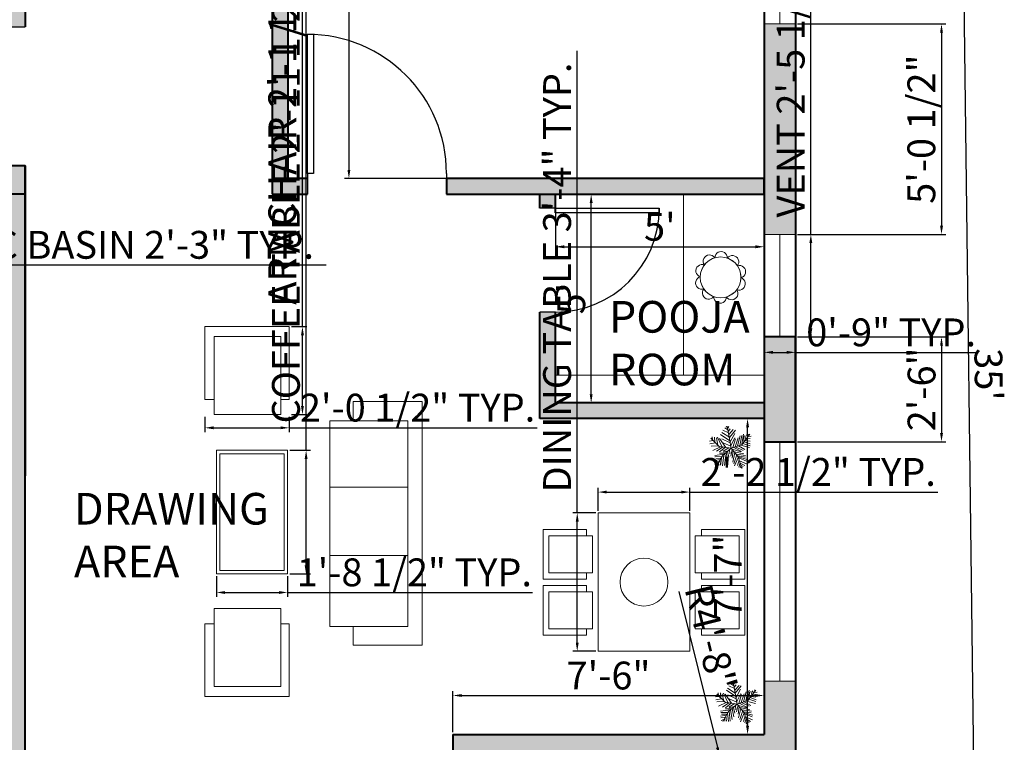
# Model space of a CAD drawing. Units: inches. Extents: x 529 to 1442, y 1029 to 1677.
# Tile 6 of 7: x 1135 to 1418, y 1252 to 1460. Entities that reach past the tile are written whole.
import ezdxf

# ---------------------------------------------------------------- set-up
doc = ezdxf.new("R2010")
doc.units = ezdxf.units.IN
for name, color, linetype, lineweight in [('A-ANNO-DIMS', 2, 'Continuous', 18), ('A-AREA-IDEN', 7, 'Continuous', 25), ('A-DOOR', 4, 'Continuous', 25), ('A-FURN', 8, 'Continuous', 18), ('A-WALL-PATT', 252, 'Continuous', 13), ('pooja', 40, 'Continuous', 18), ('tree', 70, 'Continuous', 13), ('wall', 7, 'Continuous', 40), ('window', 52, 'Continuous', 18)]:
    doc.layers.add(name, color=color, linetype=linetype, lineweight=lineweight)
doc.styles.get("Standard").update_dxf_attribs({"font": 'arial.ttf'})
doc.dimstyles.new('ISO-25', dxfattribs={"dimtxt": 8, "dimasz": 2.5, "dimexe": 1.25, "dimexo": 0.625, "dimtad": 1, "dimdec": 0, "dimlunit": 4, "dimtxsty": 'Standard', "dimcen": 2.5, "dimadec": 0, "dimazin": 0, "dimtfac": 1, "dimtdec": 0, "dimtmove": 0, "dimatfit": 3, "dimfxl": 1, "dimarcsym": 0})

# ---------------------------------------------------------------- blocks, each defined once
blk = doc.blocks.new('*U2')
for p, q in [((0, 0), (0, -6)), ((40, 0), (40, -6))]:
    blk.add_line(p, q)
blk.add_lwpolyline([(0, 0), (0, 40), (1.75, 40), (1.75, 0)], close=True)
blk.add_arc((0, 0), 40, 0, 90)
blk = doc.blocks.new('*U7')
blk.add_circle((0, -0.78), 5.87)
blk.add_arc((0.14, 4.85), 1.8, 357.1489, 180)
blk = doc.blocks.new('*U8')
at = {"layer": 'pooja', "transparency": 16777216}
for p, rotation in [((1336.39, 1386.05), 36), ((1336.39, 1384.79), 144), ((1336.11, 1385.66), 72), ((1337.31, 1386.05), 324.0000000000001), ((1337.31, 1384.79), 216), ((1337.6, 1385.66), 288), ((1336.11, 1385.18), 108), ((1337.6, 1385.18), 252), ((1336.85, 1384.64), 180)]:
    blk.add_blockref('*U7', p, dxfattribs=dict(at, rotation=rotation))
blk.add_blockref('*U7', (1336.85, 1386.2), dxfattribs=at)
blk = doc.blocks.new('*U12')
for p, q in [((-8.737, 47.138), (-17.069, 52.711)), ((-10.186, 53.64), (-13.084, 55.962)), ((0, 0), (-10.5, 57)), ((-9.099, 51.782), (-6.563, 55.962)), ((-31.5, 4.5), (-52.5, 25.5)), ((-48.585, 21.131), (-49.309, 29.026)), ((-43.513, 28.561), (-42.427, 15.558)), ((-38.442, 26.239), (-34.819, 7.663)), ((-35.544, 28.097), (-24.314, 3.947)), ((-3.665, 19.273), (-27.574, 35.527)), ((-5.114, 28.097), (-24.676, 40.636)), ((-7.288, 39.707), (-21.778, 46.673)), ((-7.65, 43.423), (-2.578, 49.46)), ((-5.839, 35.992), (4.667, 48.067)), ((-5.114, 27.632), (10.463, 46.673)), ((-2.941, 16.486), (8.652, 37.85)), ((-1.129, 6.734), (9.014, 26.704)), ((10.101, 3.483), (17.708, 26.239)), ((16.259, 5.805), (23.142, 31.348)), ((22.055, 7.198), (27.489, 32.277)), ((27, 9), (48, 36)), ((27.127, 9.056), (31.112, 35.992)), ((31.836, 30.883), (32.561, 16.486)), ((35.096, 32.741), (37.27, 22.524)), ((38.719, 34.134), (41.979, 28.561)), ((40.53, 25.775), (48.862, 24.846)), ((43.791, 29.954), (51.036, 30.883)), ((44.153, 36.456), (45.239, 32.741)), ((-47.498, 19.737), (-55.83, 18.344)), ((-40.615, 13.7), (-55.105, 10.913)), ((-33.37, 6.269), (-52.207, 5.34)), ((-28.299, 3.483), (-47.86, -5.805)), ((-21.416, 3.018), (-38.079, -8.128)), ((0, 0), (-31.5, 4.5)), ((-14.533, 2.09), (-30.834, 25.31)), ((-15.982, 2.09), (-30.11, -9.521)), ((-24.314, 23.917), (-2.941, 13.7)), ((0, 0), (-22.5, -19.5)), ((-6.563, 1.161), (-21.416, -8.128)), ((-20.691, 13.7), (-1.129, 4.876)), ((0, 0), (27, 9)), ((0, 0), (18, -22.5)), ((3.942, 1.625), (11.187, 24.381)), ((6.478, 1.625), (26.04, -8.592)), ((11.187, 3.483), (30.749, -5.805)), ((18.07, 5.805), (35.096, -3.483)), ((24.229, 7.663), (46.688, 1.625)), ((29.662, 12.307), (48.137, 6.269)), ((33.285, 16.486), (48.862, 10.913)), ((36.183, 19.737), (48.137, 17.88)), ((-17.431, -15.094), (-42.789, -18.809)), ((-24.314, -21.596), (-42.427, -22.06)), ((-22.5, -19.5), (-37.5, -45)), ((-15.257, -12.772), (-30.11, -12.772)), ((-25.038, -23.918), (-22.865, -45.281)), ((-20.691, -18.345), (-17.793, -44.352)), ((-6.563, -5.805), (-19.967, -9.985)), ((-17.069, -15.094), (-12.721, -40.172)), ((-13.446, -11.378), (-8.737, -32.741)), ((-9.461, -8.592), (-6.201, -23.453)), ((-4.752, -3.483), (-3.665, -14.629)), ((2.493, -3.019), (-1.491, -20.202)), ((1.769, -2.555), (24.229, -9.521)), ((5.029, -6.27), (2.131, -25.775)), ((9.014, -11.378), (3.58, -35.992)), ((14.085, -16.951), (6.478, -40.172)), ((7.565, -9.056), (32.198, -14.629)), ((18.07, -22.524), (8.289, -45.745)), ((12.274, -15.094), (36.907, -18.809)), ((16.259, -19.738), (36.183, -22.989)), ((18, -22.5), (27, -52.5)), ((18.433, -22.524), (40.53, -29.026)), ((19.157, -25.311), (38.719, -33.206)), ((-28.299, -29.026), (-42.789, -31.348)), ((-30.834, -34.135), (-42.427, -35.528)), ((-34.457, -39.708), (-40.978, -42.494)), ((-26.849, -26.24), (-40.253, -25.775)), ((-32.646, -36.921), (-31.921, -44.352)), ((-29.023, -30.884), (-27.936, -43.887)), ((20.244, -30.419), (15.897, -44.816)), ((22.78, -37.85), (19.519, -48.532)), ((21.331, -32.741), (39.081, -40.636)), ((22.78, -38.314), (34.372, -44.816)), ((24.591, -45.745), (23.142, -50.854)), ((24.591, -43.423), (30.749, -47.603)), ((26.764, -49.925), (28.213, -50.854))]:
    blk.add_line(p, q)
blk = doc.blocks.new('*D24')
at = {"layer": 'A-ANNO-DIMS', "color": 0, "lineweight": -2, "transparency": 16777216}
for p, q in [((1348.76, 1557.81), (1228.73, 1557.81)), ((1229.98, 1555.31), (1229.98, 1416.31)), ((1348.76, 1413.81), (1228.73, 1413.81))]:
    blk.add_line(p, q, dxfattribs=at)
at = {"layer": 'A-ANNO-DIMS', "color": 0, "lineweight": 100, "transparency": 16777216}
for points in [[(1229.56, 1555.31), (1230.39, 1555.31), (1229.98, 1557.81)], [(1229.56, 1416.31), (1230.39, 1416.31), (1229.98, 1413.81)]]:
    blk.add_solid(points, dxfattribs=at)
at = {"layer": 'Defpoints', "color": 0, "lineweight": 100, "transparency": 16777216}
for p in [(1349.38, 1557.81), (1229.98, 1413.81), (1349.38, 1413.81)]:
    blk.add_point(p, dxfattribs=at)
at = {"layer": 'A-ANNO-DIMS', "color": 0, "transparency": 16777216, "insert": (1225.34, 1485.81), "char_height": 8, "attachment_point": 5, "rotation": 90}
blk.add_mtext("12'", dxfattribs=at)
blk = doc.blocks.new('*D25')
at = {"layer": 'A-ANNO-DIMS', "color": 0, "lineweight": -2, "transparency": 16777216}
for p, q in [((1289.38, 1408.69), (1289.38, 1392.96)), ((1349.38, 1408.69), (1349.38, 1392.96)), ((1291.88, 1394.21), (1346.88, 1394.21))]:
    blk.add_line(p, q, dxfattribs=at)
at = {"layer": 'A-ANNO-DIMS', "color": 0, "lineweight": 100, "transparency": 16777216}
for points in [[(1291.88, 1394.63), (1291.88, 1393.79), (1289.38, 1394.21)], [(1346.88, 1394.63), (1346.88, 1393.79), (1349.38, 1394.21)]]:
    blk.add_solid(points, dxfattribs=at)
at = {"layer": 'Defpoints', "color": 0, "lineweight": 100, "transparency": 16777216}
for p in [(1289.38, 1409.31), (1349.38, 1409.31), (1349.38, 1394.21)]:
    blk.add_point(p, dxfattribs=at)
at = {"layer": 'A-ANNO-DIMS', "color": 0, "transparency": 16777216, "insert": (1319.38, 1398.9), "char_height": 8, "attachment_point": 5}
blk.add_mtext("5'", dxfattribs=at)
blk = doc.blocks.new('*D26')
at = {"layer": 'A-ANNO-DIMS', "color": 0, "lineweight": -2, "transparency": 16777216}
for p, q in [((1348.76, 1409.31), (1298.39, 1409.31)), ((1299.64, 1351.81), (1299.64, 1406.81)), ((1348.76, 1349.31), (1298.39, 1349.31))]:
    blk.add_line(p, q, dxfattribs=at)
at = {"layer": 'A-ANNO-DIMS', "color": 0, "lineweight": 100, "transparency": 16777216}
for points in [[(1299.22, 1406.81), (1300.06, 1406.81), (1299.64, 1409.31)], [(1299.22, 1351.81), (1300.06, 1351.81), (1299.64, 1349.31)]]:
    blk.add_solid(points, dxfattribs=at)
at = {"layer": 'Defpoints', "color": 0, "lineweight": 100, "transparency": 16777216}
for p in [(1299.64, 1409.31), (1349.38, 1409.31), (1349.38, 1349.31)]:
    blk.add_point(p, dxfattribs=at)
at = {"layer": 'A-ANNO-DIMS', "color": 0, "transparency": 16777216, "insert": (1294.95, 1379.31), "char_height": 8, "attachment_point": 5, "rotation": 90}
blk.add_mtext("5'", dxfattribs=at)
blk = doc.blocks.new('*D27')
at = {"layer": 'A-ANNO-DIMS', "color": 0, "lineweight": -2, "transparency": 16777216}
for p, q in [((1348.76, 1344.81), (1343.36, 1344.81)), ((1344.61, 1256.47), (1344.61, 1342.31)), ((1348.76, 1253.97), (1343.36, 1253.97))]:
    blk.add_line(p, q, dxfattribs=at)
at = {"layer": 'A-ANNO-DIMS', "color": 0, "lineweight": 100, "transparency": 16777216}
for points in [[(1344.19, 1342.31), (1345.03, 1342.31), (1344.61, 1344.81)], [(1344.19, 1256.47), (1345.03, 1256.47), (1344.61, 1253.97)]]:
    blk.add_solid(points, dxfattribs=at)
at = {"layer": 'Defpoints', "color": 0, "lineweight": 100, "transparency": 16777216}
for p in [(1344.61, 1344.81), (1349.38, 1344.81), (1349.38, 1253.97)]:
    blk.add_point(p, dxfattribs=at)
at = {"layer": 'A-ANNO-DIMS', "color": 0, "transparency": 16777216, "insert": (1339.98, 1299.39), "char_height": 8, "attachment_point": 5, "rotation": 90}
blk.add_mtext('7\'-7"', dxfattribs=at)
blk = doc.blocks.new('*D28')
at = {"layer": 'A-ANNO-DIMS', "color": 0, "lineweight": -2, "transparency": 16777216}
for p, q in [((1259.88, 1254.59), (1259.88, 1266.43)), ((1349.38, 1254.59), (1349.38, 1266.43)), ((1262.38, 1265.18), (1346.88, 1265.18))]:
    blk.add_line(p, q, dxfattribs=at)
at = {"layer": 'A-ANNO-DIMS', "color": 0, "lineweight": 100, "transparency": 16777216}
for points in [[(1262.38, 1265.59), (1262.38, 1264.76), (1259.88, 1265.18)], [(1346.88, 1265.59), (1346.88, 1264.76), (1349.38, 1265.18)]]:
    blk.add_solid(points, dxfattribs=at)
at = {"layer": 'Defpoints', "color": 0, "lineweight": 100, "transparency": 16777216}
for p in [(1349.38, 1265.18), (1259.88, 1253.97), (1349.38, 1253.97)]:
    blk.add_point(p, dxfattribs=at)
at = {"layer": 'A-ANNO-DIMS', "color": 0, "transparency": 16777216, "insert": (1304.63, 1269.89), "char_height": 8, "attachment_point": 5}
blk.add_mtext('7\'-6"', dxfattribs=at)
blk = doc.blocks.new('*D56')
at = {"layer": 'A-ANNO-DIMS', "color": 0, "lineweight": -2, "transparency": 16777216}
for p, q in [((1359.01, 1566.82), (1406.77, 1567.43)), ((1405.56, 1564.91), (1410.83, 1149.91)), ((1364.34, 1146.82), (1412.11, 1147.43))]:
    blk.add_line(p, q, dxfattribs=at)
at = {"layer": 'A-ANNO-DIMS', "color": 0, "lineweight": 100, "transparency": 16777216}
for points in [[(1405.97, 1564.92), (1405.14, 1564.91), (1405.52, 1567.41)], [(1411.24, 1149.92), (1410.41, 1149.91), (1410.86, 1147.41)]]:
    blk.add_solid(points, dxfattribs=at)
at = {"layer": 'Defpoints', "color": 0, "lineweight": 100, "transparency": 16777216}
for p in [(1358.38, 1566.81), (1363.72, 1146.81), (1410.86, 1147.41)]:
    blk.add_point(p, dxfattribs=at)
at = {"layer": 'A-ANNO-DIMS', "color": 0, "transparency": 16777216, "insert": (1412.9, 1357.47), "char_height": 8, "attachment_point": 5, "rotation": 270.7276}
blk.add_mtext("35'", dxfattribs=at)
blk = doc.blocks.new('WIN-LARGE-PLAN')
blk.add_line((0, 4.5), (68.85, 4.5))
blk.add_lwpolyline([(0, 9), (68.85, 9), (68.85, 0), (0, 0)], close=True)
blk = doc.blocks.new('WIN-VENT-PLAN')
blk.add_line((4.5, 0), (4.5, 29.5))
blk.add_lwpolyline([(0, 29.5), (9, 29.5), (9, 0), (0, 0)], close=True)
blk = doc.blocks.new('DINING-CHAIR')
for p, q in [((1.76, 12.47), (1.76, 14.29)), ((1.76, 14.29), (14.22, 14.29)), ((14.22, 14.29), (14.22, 0)), ((1.76, 0), (1.76, 1.83)), ((14.22, 0), (1.76, 0))]:
    blk.add_line(p, q)
blk.add_lwpolyline([(0, 12.47), (12.59, 12.47), (12.59, 1.83), (0, 1.83)], close=True)
blk = doc.blocks.new('DINING-TABLE')
blk.add_lwpolyline([(26.42, 39.82), (0, 39.82), (0, 0), (26.42, 0)], close=True)
blk.add_circle((13.21, 19.91), 6.89)
blk = doc.blocks.new('SOFA-THREE-SEAT')
for p, q in [((6.71, 64.51), (6.71, 70.05)), ((6.71, 70.05), (26.55, 70.05)), ((26.55, 70.05), (26.55, 0)), ((0, 45.39), (22.47, 45.39)), ((0, 25.77), (22.47, 25.77)), ((6.71, 0), (6.71, 5.33)), ((26.55, 0), (6.71, 0))]:
    blk.add_line(p, q)
for points in [[(22.47, 64.51), (0, 64.51), (0, 5.33), (22.47, 5.33)], [(0, 45.39), (22.47, 45.39), (22.47, 64.51), (0, 64.51)]]:
    blk.add_lwpolyline(points, close=True)
blk = doc.blocks.new('LOUNGE-CHAIR')
for p, q in [((0, 4.37), (0, 25.3)), ((0, 25.3), (24.27, 25.3)), ((24.27, 25.3), (24.27, 4.37)), ((2.68, 4.37), (0, 4.37)), ((2.68, 4.37), (2.68, 4.37)), ((24.27, 4.37), (21.8, 4.37))]:
    blk.add_line(p, q)
blk.add_lwpolyline([(2.68, 22.46), (2.68, 0), (21.8, 0), (21.8, 22.46)], close=True)
blk = doc.blocks.new('COFFEE-TABLE')
for points in [[(0, 35.56), (20.45, 35.56), (20.45, 0), (0, 0)], [(1, 34.56), (19.45, 34.56), (19.45, 1), (1, 1)]]:
    blk.add_lwpolyline(points, close=True)
blk = doc.blocks.new('*D75')
at = {"layer": 'A-ANNO-DIMS', "color": 0, "lineweight": -2, "transparency": 16777216}
for p, q in [((1362.81, 1397.77), (1362.81, 1502.25)), ((1359.01, 1397.77), (1364.06, 1397.77)), ((1362.81, 1370.77), (1362.81, 1395.27)), ((1359.01, 1368.27), (1364.06, 1368.27))]:
    blk.add_line(p, q, dxfattribs=at)
at = {"layer": 'A-ANNO-DIMS', "color": 0, "lineweight": 100, "transparency": 16777216}
for points in [[(1362.39, 1395.27), (1363.23, 1395.27), (1362.81, 1397.77)], [(1362.39, 1370.77), (1363.23, 1370.77), (1362.81, 1368.27)]]:
    blk.add_solid(points, dxfattribs=at)
at = {"layer": 'Defpoints', "color": 0, "lineweight": 100, "transparency": 16777216}
for p in [(1358.38, 1397.77), (1362.81, 1397.77), (1358.38, 1368.27)]:
    blk.add_point(p, dxfattribs=at)
at = {"layer": 'A-ANNO-DIMS', "color": 0, "transparency": 16777216, "insert": (1358.05, 1451.26), "char_height": 8, "attachment_point": 5, "rotation": 90}
blk.add_mtext('VENT 2\'-5 1/2" TYP.', dxfattribs=at)
blk = doc.blocks.new('*D76')
at = {"layer": 'A-ANNO-DIMS', "color": 0, "lineweight": -2, "transparency": 16777216}
for p, q in [((1349.38, 1367.65), (1349.38, 1362.6)), ((1358.38, 1367.65), (1358.38, 1362.6)), ((1351.88, 1363.85), (1355.88, 1363.85)), ((1358.38, 1363.85), (1410.9, 1363.85))]:
    blk.add_line(p, q, dxfattribs=at)
at = {"layer": 'A-ANNO-DIMS', "color": 0, "lineweight": 100, "transparency": 16777216}
for points in [[(1351.88, 1364.26), (1351.88, 1363.43), (1349.38, 1363.85)], [(1355.88, 1364.26), (1355.88, 1363.43), (1358.38, 1363.85)]]:
    blk.add_solid(points, dxfattribs=at)
at = {"layer": 'Defpoints', "color": 0, "lineweight": 100, "transparency": 16777216}
for p in [(1349.38, 1368.27), (1358.38, 1368.27), (1358.38, 1363.85)]:
    blk.add_point(p, dxfattribs=at)
at = {"layer": 'A-ANNO-DIMS', "color": 0, "transparency": 16777216, "insert": (1385.89, 1368.56), "char_height": 8, "attachment_point": 5}
blk.add_mtext('0\'-9" TYP.', dxfattribs=at)
blk = doc.blocks.new('*D77')
at = {"layer": 'A-ANNO-DIMS', "color": 0, "lineweight": -2, "transparency": 16777216}
for p, q in [((1262.64, 1475.94), (1262.64, 1462.3)), ((1349.38, 1475.94), (1349.38, 1462.3)), ((1262.64, 1463.55), (1116.74, 1463.55)), ((1346.88, 1463.55), (1265.14, 1463.55))]:
    blk.add_line(p, q, dxfattribs=at)
at = {"layer": 'A-ANNO-DIMS', "color": 0, "lineweight": 100, "transparency": 16777216}
for points in [[(1265.14, 1463.97), (1265.14, 1463.13), (1262.64, 1463.55)], [(1346.88, 1463.97), (1346.88, 1463.13), (1349.38, 1463.55)]]:
    blk.add_solid(points, dxfattribs=at)
at = {"layer": 'Defpoints', "color": 0, "lineweight": 100, "transparency": 16777216}
for p in [(1262.64, 1476.56), (1349.38, 1476.56), (1262.64, 1463.55)]:
    blk.add_point(p, dxfattribs=at)
at = {"layer": 'A-ANNO-DIMS', "color": 0, "transparency": 16777216, "insert": (1188.44, 1468.32), "char_height": 8, "attachment_point": 5}
blk.add_mtext('DOUBLE BED 7\'-2 1/2" TYP.', dxfattribs=at)
blk = doc.blocks.new('*D83')
at = {"layer": 'A-ANNO-DIMS', "color": 0, "lineweight": -2, "transparency": 16777216}
for p, q in [((1295.63, 1317.7), (1295.63, 1450.55)), ((1300.98, 1317.7), (1294.38, 1317.7)), ((1295.63, 1280.38), (1295.63, 1315.2)), ((1300.98, 1277.88), (1294.38, 1277.88))]:
    blk.add_line(p, q, dxfattribs=at)
at = {"layer": 'A-ANNO-DIMS', "color": 0, "lineweight": 100, "transparency": 16777216}
for points in [[(1295.22, 1315.2), (1296.05, 1315.2), (1295.63, 1317.7)], [(1295.22, 1280.38), (1296.05, 1280.38), (1295.63, 1277.88)]]:
    blk.add_solid(points, dxfattribs=at)
at = {"layer": 'Defpoints', "color": 0, "lineweight": 100, "transparency": 16777216}
for p in [(1295.63, 1317.7), (1301.61, 1317.7), (1301.61, 1277.88)]:
    blk.add_point(p, dxfattribs=at)
at = {"layer": 'A-ANNO-DIMS', "color": 0, "transparency": 16777216, "insert": (1290.87, 1385.37), "char_height": 8, "attachment_point": 5, "rotation": 90}
blk.add_mtext('DINING TABLE 3\'-4" TYP.', dxfattribs=at)
blk = doc.blocks.new('*D84')
at = {"layer": 'A-ANNO-DIMS', "color": 0, "lineweight": -2, "transparency": 16777216}
for p, q in [((1301.61, 1318.32), (1301.61, 1324.92)), ((1304.11, 1323.67), (1325.53, 1323.67)), ((1328.03, 1318.32), (1328.03, 1324.92)), ((1328.03, 1323.67), (1399.32, 1323.67))]:
    blk.add_line(p, q, dxfattribs=at)
at = {"layer": 'A-ANNO-DIMS', "color": 0, "lineweight": 100, "transparency": 16777216}
for points in [[(1304.11, 1324.09), (1304.11, 1323.26), (1301.61, 1323.67)], [(1325.53, 1324.09), (1325.53, 1323.26), (1328.03, 1323.67)]]:
    blk.add_solid(points, dxfattribs=at)
at = {"layer": 'Defpoints', "color": 0, "lineweight": 100, "transparency": 16777216}
for p in [(1328.03, 1323.67), (1301.61, 1317.7), (1328.03, 1317.7)]:
    blk.add_point(p, dxfattribs=at)
at = {"layer": 'A-ANNO-DIMS', "color": 0, "transparency": 16777216, "insert": (1364.92, 1328.43), "char_height": 8, "attachment_point": 5}
blk.add_mtext('2\'-2 1/2" TYP.', dxfattribs=at)
blk = doc.blocks.new('*D85')
at = {"layer": 'A-ANNO-DIMS', "color": 0, "lineweight": -2, "transparency": 16777216}
for p, q in [((1085.24, 1392.4), (1085.24, 1387.72)), ((1112.26, 1392.4), (1112.26, 1387.72)), ((1087.74, 1388.97), (1109.76, 1388.97)), ((1112.26, 1388.97), (1223.47, 1388.97))]:
    blk.add_line(p, q, dxfattribs=at)
at = {"layer": 'A-ANNO-DIMS', "color": 0, "lineweight": 100, "transparency": 16777216}
for points in [[(1087.74, 1389.38), (1087.74, 1388.55), (1085.24, 1388.97)], [(1109.76, 1389.38), (1109.76, 1388.55), (1112.26, 1388.97)]]:
    blk.add_solid(points, dxfattribs=at)
at = {"layer": 'Defpoints', "color": 0, "lineweight": 100, "transparency": 16777216}
for p in [(1085.24, 1393.02), (1112.26, 1393.02), (1112.26, 1388.97)]:
    blk.add_point(p, dxfattribs=at)
at = {"layer": 'A-ANNO-DIMS', "color": 0, "transparency": 16777216, "insert": (1169.11, 1393.73), "char_height": 8, "attachment_point": 5}
blk.add_mtext('WC BASIN 2\'-3" TYP.', dxfattribs=at)
blk = doc.blocks.new('*D87')
at = {"layer": 'A-ANNO-DIMS', "color": 0, "lineweight": -2, "transparency": 16777216}
for p, q in [((1216.62, 1371.24), (1216.62, 1505.58)), ((1213.45, 1371.24), (1217.87, 1371.24)), ((1216.62, 1348.45), (1216.62, 1368.74)), ((1213.45, 1345.95), (1217.87, 1345.95))]:
    blk.add_line(p, q, dxfattribs=at)
at = {"layer": 'A-ANNO-DIMS', "color": 0, "lineweight": 100, "transparency": 16777216}
for points in [[(1216.2, 1368.74), (1217.04, 1368.74), (1216.62, 1371.24)], [(1216.2, 1348.45), (1217.04, 1348.45), (1216.62, 1345.95)]]:
    blk.add_solid(points, dxfattribs=at)
at = {"layer": 'Defpoints', "color": 0, "lineweight": 100, "transparency": 16777216}
for p in [(1212.83, 1371.24), (1216.62, 1371.24), (1212.83, 1345.95)]:
    blk.add_point(p, dxfattribs=at)
at = {"layer": 'A-ANNO-DIMS', "color": 0, "transparency": 16777216, "insert": (1211.86, 1439.66), "char_height": 8, "attachment_point": 5, "rotation": 90}
blk.add_mtext('ARMCHAIR 2\'-1 1/2" TYP.', dxfattribs=at)
blk = doc.blocks.new('*D88')
at = {"layer": 'A-ANNO-DIMS', "color": 0, "lineweight": -2, "transparency": 16777216}
for p, q in [((1188.56, 1345.32), (1188.56, 1340.9)), ((1212.83, 1345.32), (1212.83, 1340.9)), ((1191.06, 1342.15), (1210.33, 1342.15)), ((1212.83, 1342.15), (1284.12, 1342.15))]:
    blk.add_line(p, q, dxfattribs=at)
at = {"layer": 'A-ANNO-DIMS', "color": 0, "lineweight": 100, "transparency": 16777216}
for points in [[(1191.06, 1342.57), (1191.06, 1341.74), (1188.56, 1342.15)], [(1210.33, 1342.57), (1210.33, 1341.74), (1212.83, 1342.15)]]:
    blk.add_solid(points, dxfattribs=at)
at = {"layer": 'Defpoints', "color": 0, "lineweight": 100, "transparency": 16777216}
for p in [(1188.56, 1345.95), (1212.83, 1345.95), (1212.83, 1342.15)]:
    blk.add_point(p, dxfattribs=at)
at = {"layer": 'A-ANNO-DIMS', "color": 0, "transparency": 16777216, "insert": (1249.72, 1346.92), "char_height": 8, "attachment_point": 5}
blk.add_mtext('2\'-0 1/2" TYP.', dxfattribs=at)
blk = doc.blocks.new('*D91')
at = {"layer": 'A-ANNO-DIMS', "color": 0, "lineweight": -2, "transparency": 16777216}
for p, q in [((1217.67, 1335.7), (1217.67, 1499.91)), ((1212.96, 1335.7), (1218.92, 1335.7)), ((1217.67, 1302.63), (1217.67, 1333.2)), ((1212.96, 1300.13), (1218.92, 1300.13))]:
    blk.add_line(p, q, dxfattribs=at)
at = {"layer": 'A-ANNO-DIMS', "color": 0, "lineweight": 100, "transparency": 16777216}
for points in [[(1217.25, 1333.2), (1218.08, 1333.2), (1217.67, 1335.7)], [(1217.25, 1302.63), (1218.08, 1302.63), (1217.67, 1300.13)]]:
    blk.add_solid(points, dxfattribs=at)
at = {"layer": 'Defpoints', "color": 0, "lineweight": 100, "transparency": 16777216}
for p in [(1212.33, 1335.7), (1217.67, 1335.7), (1212.33, 1300.13)]:
    blk.add_point(p, dxfattribs=at)
at = {"layer": 'A-ANNO-DIMS', "color": 0, "transparency": 16777216, "insert": (1212.9, 1419.05), "char_height": 8, "attachment_point": 5, "rotation": 90}
blk.add_mtext('COFFEE TABLE 2\'-11 1/2" TYP.', dxfattribs=at)
blk = doc.blocks.new('*D92')
at = {"layer": 'A-ANNO-DIMS', "color": 0, "lineweight": -2, "transparency": 16777216}
for p, q in [((1191.89, 1299.51), (1191.89, 1293.55)), ((1212.33, 1299.51), (1212.33, 1293.55)), ((1194.39, 1294.8), (1209.83, 1294.8)), ((1212.33, 1294.8), (1282.74, 1294.8))]:
    blk.add_line(p, q, dxfattribs=at)
at = {"layer": 'A-ANNO-DIMS', "color": 0, "lineweight": 100, "transparency": 16777216}
for points in [[(1194.39, 1295.21), (1194.39, 1294.38), (1191.89, 1294.8)], [(1209.83, 1295.21), (1209.83, 1294.38), (1212.33, 1294.8)]]:
    blk.add_solid(points, dxfattribs=at)
at = {"layer": 'Defpoints', "color": 0, "lineweight": 100, "transparency": 16777216}
for p in [(1191.89, 1300.13), (1212.33, 1300.13), (1212.33, 1294.8)]:
    blk.add_point(p, dxfattribs=at)
at = {"layer": 'A-ANNO-DIMS', "color": 0, "transparency": 16777216, "insert": (1248.78, 1299.56), "char_height": 8, "attachment_point": 5}
blk.add_mtext('1\'-8 1/2" TYP.', dxfattribs=at)
blk = doc.blocks.new('*D109')
at = {"layer": 'A-ANNO-DIMS', "color": 0, "lineweight": -2, "transparency": 16777216}
for p, q in [((1359.01, 1458.28), (1401.63, 1458.28)), ((1400.38, 1455.78), (1400.38, 1400.27)), ((1359.01, 1397.77), (1401.63, 1397.77))]:
    blk.add_line(p, q, dxfattribs=at)
at = {"layer": 'A-ANNO-DIMS', "color": 0, "lineweight": 100, "transparency": 16777216}
for points in [[(1399.97, 1455.78), (1400.8, 1455.78), (1400.38, 1458.28)], [(1399.97, 1400.27), (1400.8, 1400.27), (1400.38, 1397.77)]]:
    blk.add_solid(points, dxfattribs=at)
at = {"layer": 'Defpoints', "color": 0, "lineweight": 100, "transparency": 16777216}
for p in [(1358.38, 1458.28), (1358.38, 1397.77), (1400.38, 1397.77)]:
    blk.add_point(p, dxfattribs=at)
at = {"layer": 'A-ANNO-DIMS', "color": 0, "transparency": 16777216, "insert": (1395.62, 1428.03), "char_height": 8, "attachment_point": 5, "rotation": 90}
blk.add_mtext('5\'-0 1/2"', dxfattribs=at)
blk = doc.blocks.new('*D110')
at = {"layer": 'A-ANNO-DIMS', "color": 0, "lineweight": -2, "transparency": 16777216}
for p, q in [((1359.01, 1368.27), (1401.63, 1368.27)), ((1400.38, 1365.77), (1400.38, 1340.65)), ((1359.01, 1338.15), (1401.63, 1338.15))]:
    blk.add_line(p, q, dxfattribs=at)
at = {"layer": 'A-ANNO-DIMS', "color": 0, "lineweight": 100, "transparency": 16777216}
for points in [[(1399.97, 1365.77), (1400.8, 1365.77), (1400.38, 1368.27)], [(1399.97, 1340.65), (1400.8, 1340.65), (1400.38, 1338.15)]]:
    blk.add_solid(points, dxfattribs=at)
at = {"layer": 'Defpoints', "color": 0, "lineweight": 100, "transparency": 16777216}
for p in [(1358.38, 1368.27), (1358.38, 1338.15), (1400.38, 1338.15)]:
    blk.add_point(p, dxfattribs=at)
at = {"layer": 'A-ANNO-DIMS', "color": 0, "transparency": 16777216, "insert": (1395.67, 1353.21), "char_height": 8, "attachment_point": 5, "rotation": 90}
blk.add_mtext('2\'-6"', dxfattribs=at)
blk = doc.blocks.new('*D117')
at = {"layer": 'A-ANNO-DIMS', "color": 0, "lineweight": -2, "transparency": 16777216}
for p, q in [((1324.84, 1295.1), (1335.92, 1250.26)), ((1349.96, 1193.47), (1336.52, 1247.84))]:
    blk.add_line(p, q, dxfattribs=at)
at = {"layer": 'A-ANNO-DIMS', "color": 0, "lineweight": 100, "transparency": 16777216}
blk.add_solid([(1336.33, 1250.36), (1335.52, 1250.16), (1336.52, 1247.84)], dxfattribs=at)
at = {"layer": 'Defpoints', "color": 0, "lineweight": 100, "transparency": 16777216}
for p in [(1336.52, 1247.84), (1349.96, 1193.47)]:
    blk.add_point(p, dxfattribs=at)
at = {"layer": 'A-ANNO-DIMS', "color": 0, "transparency": 16777216, "insert": (1333.03, 1281.58), "char_height": 8, "attachment_point": 5, "rotation": 283.8857}
blk.add_mtext('R4\'-8"', dxfattribs=at)

msp = doc.modelspace()

# ---------------------------------------------------------------- hatches: boundary and pattern name
at = {"layer": 'A-WALL-PATT'}
h = msp.add_hatch(color=256, dxfattribs=at)
h.dxf.hatch_style = 1
h.paths.add_polyline_path([(1160.38, 1566.81), (1099.95, 1566.81), (1099.95, 1557.81), (1132.38, 1557.81), (1160.38, 1557.81)])
h.paths.add_polyline_path([(1136.88, 1557.81), (1132.38, 1557.81), (1132.38, 1457.46), (1136.88, 1457.46)])
h.paths.add_polyline_path([(1171.8, 1467.81), (1136.88, 1467.81), (1136.88, 1463.31), (1171.8, 1463.31)])
h.paths.add_polyline_path([(1212.38, 1557.81), (1207.88, 1557.81), (1207.88, 1467.81), (1207.88, 1409.31), (1218.04, 1409.31), (1218.04, 1413.81), (1212.38, 1413.81), (1212.38, 1463.31)])
h.paths.add_polyline_path([(1136.88, 1409.31), (1132.38, 1409.31), (1132.38, 1146.81), (1136.88, 1146.81)])
h.paths.add_polyline_path([(1136.88, 1417.46), (1132.38, 1417.46), (1132.38, 1409.31), (1136.88, 1409.31)])
h.paths.add_polyline_path([(1132.38, 1413.81), (1075.12, 1413.81), (1075.12, 1409.31), (1132.38, 1409.31)])
h.paths.add_polyline_path([(1132.38, 1328.31), (1041.38, 1328.31), (1041.38, 1323.81), (1132.38, 1323.81)])
h = msp.add_hatch(color=256, dxfattribs=at)
h.dxf.hatch_style = 1
h.paths.add_polyline_path([(1171.8, 1467.81), (1136.88, 1467.81), (1136.88, 1463.31), (1171.8, 1463.31)])
h.paths.add_polyline_path([(1136.88, 1557.81), (1132.38, 1557.81), (1132.38, 1457.46), (1136.88, 1457.46)])
h.paths.add_polyline_path([(1212.38, 1557.81), (1207.88, 1557.81), (1207.88, 1467.81), (1207.88, 1409.31), (1218.04, 1409.31), (1218.04, 1413.81), (1212.38, 1413.81), (1212.38, 1463.31)])
h = msp.add_hatch(color=256, dxfattribs=at)
h.dxf.hatch_style = 1
h.paths.add_polyline_path([(1358.38, 1368.27), (1349.38, 1368.27), (1349.38, 1338.15), (1358.38, 1338.15)])
h.paths.add_polyline_path([(1349.38, 1349.31), (1289.38, 1349.31), (1289.38, 1375.44), (1284.88, 1375.44), (1284.88, 1344.81), (1349.38, 1344.81)])
h.paths.add_polyline_path([(1358.38, 1458.28), (1349.38, 1458.28), (1349.38, 1413.81), (1349.38, 1397.77), (1358.38, 1397.77)])
h.paths.add_polyline_path([(1289.38, 1409.31), (1284.88, 1409.31), (1284.88, 1405.28), (1289.38, 1405.28)])
h = msp.add_hatch(color=256, dxfattribs=at)
h.dxf.hatch_style = 1
h.paths.add_polyline_path([(1259.88, 1228.31), (1187.26, 1228.31), (1187.26, 1226.94), (1187.26, 1223.81), (1259.88, 1223.81)])
h.paths.add_polyline_path([(1145.62, 1226.94), (1145.62, 1228.31), (1136.88, 1228.31), (1136.88, 1223.81), (1145.62, 1223.81)])
h.paths.add_polyline_path([(1136.88, 1228.31), (1132.38, 1228.31), (1132.38, 1146.81), (1136.88, 1146.81)])
h.paths.add_polyline_path([(1136.88, 1417.46), (1132.38, 1417.46), (1132.38, 1228.31), (1136.88, 1228.31)])
h = msp.add_hatch(color=256, dxfattribs=at)
h.dxf.hatch_style = 1
h.paths.add_polyline_path([(1349.38, 1413.81), (1258.04, 1413.81), (1258.04, 1409.31), (1349.38, 1409.31)])
h = msp.add_hatch(color=256, dxfattribs=at)
h.dxf.hatch_style = 1
h.paths.add_polyline_path([(1292.57, 1155.81), (1264.38, 1155.81), (1264.38, 1146.81), (1292.57, 1146.81)], flags=17)
h.paths.add_polyline_path([(1358.38, 1269.29), (1349.38, 1269.29), (1349.38, 1259.81), (1349.38, 1155.81), (1323.86, 1155.81), (1323.86, 1146.81), (1358.38, 1146.81)])
h.paths.add_polyline_path([(1264.38, 1249.47), (1349.38, 1249.47), (1349.38, 1253.97), (1259.88, 1253.97), (1259.88, 1164.81), (1259.88, 1146.81), (1264.38, 1146.81), (1264.38, 1155.81)])

# ---------------------------------------------------------------- linework, layer by layer
at = {"layer": 'pooja'}
msp.add_line((1289.38, 1357.28), (1349.38, 1357.28), dxfattribs=at)
msp.add_lwpolyline([(1326.22, 1357.28), (1349.38, 1357.28), (1349.38, 1409.31), (1326.22, 1409.31)], close=True, dxfattribs=at)
at = {"layer": 'wall'}
for p, q in [((1358.38, 1566.81), (1358.38, 1146.81)), ((1349.38, 1557.81), (1349.38, 1413.81)), ((1207.88, 1467.81), (1207.88, 1409.31)), ((1136.88, 1463.31), (1136.88, 1457.46)), ((1212.38, 1463.31), (1212.38, 1413.81)), ((1136.88, 1417.46), (1136.88, 1409.31)), ((1218.04, 1413.81), (1212.38, 1413.81)), ((1349.38, 1413.81), (1258.04, 1413.81)), ((1136.88, 1409.31), (1075.12, 1409.31)), ((1136.88, 1409.31), (1136.88, 1328.31)), ((1207.88, 1409.31), (1218.04, 1409.31)), ((1258.04, 1409.31), (1349.38, 1409.31)), ((1284.88, 1405.28), (1284.88, 1409.31)), ((1289.38, 1403.98), (1289.38, 1409.31)), ((1349.38, 1409.31), (1349.38, 1349.31)), ((1284.88, 1344.81), (1284.88, 1375.44)), ((1289.38, 1349.31), (1289.38, 1375.44)), ((1349.38, 1349.31), (1289.38, 1349.31)), ((1349.38, 1344.81), (1284.88, 1344.81)), ((1349.38, 1344.81), (1349.38, 1259.81)), ((1136.88, 1164.81), (1136.88, 1328.31)), ((1259.88, 1253.97), (1259.88, 1164.81)), ((1259.88, 1253.97), (1349.38, 1253.97))]:
    msp.add_line(p, q, dxfattribs=at)
for points in [[(859.38, 1146.81), (638.38, 1146.81), (638.38, 1566.81), (1358.38, 1566.81), (1358.38, 1146.81), (1132.38, 1146.81)], [(1212.38, 1557.81), (1349.38, 1557.81), (1349.38, 1253.97)]]:
    msp.add_lwpolyline(points, dxfattribs=at)
for points in [[(1132.38, 1146.81), (1136.88, 1146.81), (1136.88, 1417.46), (1132.38, 1417.46)], [(1258.04, 1409.31), (1349.38, 1409.31), (1349.38, 1413.81), (1258.04, 1413.81)], [(1349.38, 1338.15), (1358.38, 1338.15), (1358.38, 1368.27), (1349.38, 1368.27)]]:
    msp.add_lwpolyline(points, close=True, dxfattribs=at)

# ---------------------------------------------------------------- block references
at = {"layer": 'A-DOOR', "rotation": 90}
msp.add_blockref('*U2', (1130.88, 1417.46), dxfattribs=at)
at = {"layer": 'A-DOOR'}
msp.add_blockref('*U2', (1218.04, 1415.31), dxfattribs=at)
at = {"layer": 'A-DOOR', "xscale": 0.7461367546467864, "yscale": 0.7461367546467864, "zscale": 0.7461367546467864, "rotation": 270}
msp.add_blockref('*U2', (1289.36, 1405.28), dxfattribs=at)
at = {"layer": 'A-FURN'}
for name, p in [('LOUNGE-CHAIR', (1188.56, 1345.95)), ('SOFA-THREE-SEAT', (1224.47, 1279.69)), ('COFFEE-TABLE', (1191.89, 1300.13)), ('DINING-TABLE', (1301.61, 1277.88)), ('DINING-CHAIR', (1329.59, 1298.59)), ('DINING-CHAIR', (1329.59, 1282.5))]:
    msp.add_blockref(name, p, dxfattribs=at)
at = {"layer": 'A-FURN', "extrusion": (0, 0, -1), "zscale": -1}
for p in [(-1300.04, 1298.59), (-1300.04, 1282.5)]:
    msp.add_blockref('DINING-CHAIR', p, dxfattribs=at)
at = {"layer": 'A-FURN', "extrusion": (0, 0, -1), "zscale": -1, "rotation": 180}
msp.add_blockref('LOUNGE-CHAIR', (-1188.56, 1290.18), dxfattribs=at)
at = {"layer": 'pooja'}
msp.add_blockref('*U8', (0, 0), dxfattribs=at)
at = {"layer": 'tree', "xscale": 0.1116431773080361, "yscale": 0.1116431773080361, "zscale": 0.1116431773080361}
for p in [(1339.94, 1336.3), (1341.64, 1262.73)]:
    msp.add_blockref('*U12', p, dxfattribs=at)
at = {"layer": 'window', "rotation": 269.9999999999987}
for p in [(1349.38, 1527.14), (1349.38, 1338.15)]:
    msp.add_blockref('WIN-LARGE-PLAN', p, dxfattribs=at)
at = {"layer": 'window'}
msp.add_blockref('WIN-VENT-PLAN', (1349.38, 1368.27), dxfattribs=at)

# ---------------------------------------------------------------- texts
at = {"layer": 'A-AREA-IDEN', "char_height": 9.098, "attachment_point": 1}
for s, insert in [('POOJA\\PROOM', (1304.76, 1378.62)), ('DRAWING\\PAREA', (1150.92, 1323.43))]:
    msp.add_mtext_dynamic_manual_height_columns(s, width=307.5887, gutter_width=45.49, heights=[0], dxfattribs=dict(at, insert=insert))

# ---------------------------------------------------------------- dimensions: what is measured, and where the dimension line sits
at = {"layer": 'A-ANNO-DIMS'}
dim = msp.add_aligned_dim(p1=(1358.38, 1566.81), p2=(1363.72, 1146.81), distance=47.14, dimstyle='ISO-25', override={"dimclrd": 0, "dimclre": 0, "dimclrt": 0}, dxfattribs=at)
dim.commit()
dim.dimension.update_dxf_attribs({"geometry": '*D56', "text_midpoint": (1412.9, 1357.47)})
for base, p1, p2, override, picture, middle in [((1229.98, 1413.81), (1349.38, 1557.81), (1349.38, 1413.81), {"dimclrd": 0, "dimclre": 0, "dimclrt": 0}, '*D24', (1225.34, 1485.81)), ((1400.38, 1397.77), (1358.38, 1458.28), (1358.38, 1397.77), {"dimdec": 1, "dimlfac": 1, "dimrnd": 0, "dimzin": 1, "dimdsep": 46, "dimlunit": 4, "dimfrac": 2}, '*D109', (1395.62, 1428.03)), ((1299.64, 1409.31), (1349.38, 1349.31), (1349.38, 1409.31), {"dimclrd": 0, "dimclre": 0, "dimclrt": 0}, '*D26', (1294.95, 1379.31)), ((1400.38, 1338.15), (1358.38, 1368.27), (1358.38, 1338.15), {"dimdec": 1, "dimlfac": 1, "dimrnd": 0, "dimzin": 1, "dimdsep": 46, "dimlunit": 4, "dimfrac": 2}, '*D110', (1395.67, 1353.21)), ((1344.61, 1344.81), (1349.38, 1253.97), (1349.38, 1344.81), {"dimclrd": 0, "dimclre": 0, "dimclrt": 0}, '*D27', (1339.98, 1299.39))]:
    dim = msp.add_linear_dim(base=base, p1=p1, p2=p2, angle=90, dimstyle='ISO-25', override=override, dxfattribs=at)
    dim.commit()
    dim.dimension.update_dxf_attribs({"geometry": picture, "text_midpoint": middle})
for base, p1, p2, angle, text, picture, middle in [((1216.62, 1371.24), (1212.83, 1345.95), (1212.83, 1371.24), 90, 'ARMCHAIR <> TYP.', '*D87', (1211.86, 1439.66)), ((1362.81, 1397.77), (1358.38, 1368.27), (1358.38, 1397.77), 90, 'VENT <> TYP.', '*D75', (1358.05, 1451.26)), ((1262.64, 1463.55), (1349.38, 1476.56), (1262.64, 1476.56), 180, 'DOUBLE BED <> TYP.', '*D77', (1188.44, 1468.32)), ((1217.67, 1335.7), (1212.33, 1300.13), (1212.33, 1335.7), 90, 'COFFEE TABLE <> TYP.', '*D91', (1212.9, 1419.05)), ((1295.63, 1317.7), (1301.61, 1277.88), (1301.61, 1317.7), 90, 'DINING TABLE <> TYP.', '*D83', (1290.87, 1385.37))]:
    dim = msp.add_linear_dim(base=base, p1=p1, p2=p2, angle=angle, text=text, dimstyle='ISO-25', override={"dimdec": 1, "dimlfac": 1, "dimrnd": 0, "dimzin": 1, "dimdsep": 46, "dimlunit": 4, "dimfrac": 2}, dxfattribs=at)
    dim.commit()
    dim.dimension.update_dxf_attribs({"geometry": picture, "text_midpoint": middle})
for base, p1, p2, text, picture, middle in [((1112.26, 1388.97), (1085.24, 1393.02), (1112.26, 1393.02), 'WC BASIN <> TYP.', '*D85', (1169.11, 1393.73)), ((1358.38, 1363.85), (1349.38, 1368.27), (1358.38, 1368.27), '<> TYP.', '*D76', (1385.89, 1368.56)), ((1212.83, 1342.15), (1188.56, 1345.95), (1212.83, 1345.95), '<> TYP.', '*D88', (1249.72, 1346.92)), ((1328.03, 1323.67), (1301.61, 1317.7), (1328.03, 1317.7), '<> TYP.', '*D84', (1364.92, 1328.43)), ((1212.33, 1294.8), (1191.89, 1300.13), (1212.33, 1300.13), '<> TYP.', '*D92', (1248.78, 1299.56))]:
    dim = msp.add_linear_dim(base=base, p1=p1, p2=p2, text=text, dimstyle='ISO-25', override={"dimdec": 1, "dimlfac": 1, "dimrnd": 0, "dimzin": 1, "dimdsep": 46, "dimlunit": 4, "dimfrac": 2}, dxfattribs=at)
    dim.commit()
    dim.dimension.update_dxf_attribs({"geometry": picture, "text_midpoint": middle})
for base, p1, p2, picture, middle in [((1349.38, 1394.21), (1289.38, 1409.31), (1349.38, 1409.31), '*D25', (1319.38, 1398.9)), ((1349.38418487, 1265.17614371), (1259.88418487, 1253.96861787), (1349.38418487, 1253.96861787), '*D28', (1304.63418487, 1269.88572762))]:
    dim = msp.add_linear_dim(base=base, p1=p1, p2=p2, dimstyle='ISO-25', override={"dimclrd": 0, "dimclre": 0, "dimclrt": 0}, dxfattribs=at)
    dim.commit()
    dim.dimension.update_dxf_attribs({"geometry": picture, "text_midpoint": middle})
dim = msp.add_radius_dim(center=(1349.96, 1193.47), mpoint=(1336.52, 1247.84), dimstyle='ISO-25', override={"dimdec": 1, "dimlfac": 1, "dimrnd": 0, "dimzin": 1, "dimdsep": 46, "dimlunit": 4, "dimfrac": 2}, dxfattribs=at)
dim.commit()
dim.dimension.update_dxf_attribs({"geometry": '*D117', "text_midpoint": (1328.46, 1280.45), "dimtype": 164})

doc.saveas('drawing.dxf')
